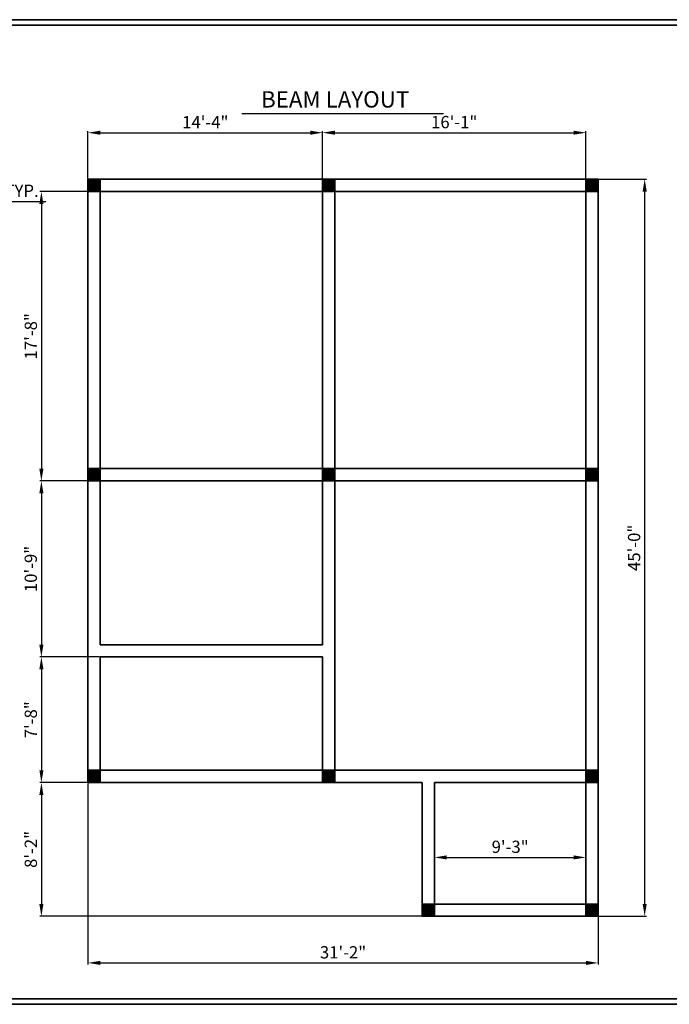
# Model space of a CAD drawing. Units: inches. Extents: x 2396 to 4051, y 1419 to 2191.
# Tile 6 of 7: x 2981 to 3457, y 1470 to 2191. Entities that reach past the tile are written whole.
import ezdxf

# ---------------------------------------------------------------- set-up
doc = ezdxf.new("R2010")
doc.units = ezdxf.units.IN
for name, color, linetype, lineweight in [('A-ANNO-TITL', 7, 'Continuous', 25), ('A-ANNO-TTLB', 7, 'Continuous', 35), ('S-ANNO-DIMS', 2, 'Continuous', 18), ('S-BEAM', 7, 'Continuous', 35)]:
    doc.layers.add(name, color=color, linetype=linetype, lineweight=lineweight)
doc.layers.add('S-COLS', color=242, linetype='Continuous', lineweight=35, true_color=0xcd2027)
doc.styles.get("Standard").update_dxf_attribs({"font": 'arial.ttf'})
doc.dimstyles.new('ISO-25', dxfattribs={"dimtxt": 9, "dimasz": 9, "dimexe": 1.25, "dimexo": 0.625, "dimgap": 2, "dimtad": 1, "dimdec": 1, "dimlunit": 4, "dimtxsty": 'Standard', "dimcen": 2.5, "dimadec": 0, "dimazin": 0, "dimtfac": 1, "dimtdec": 1, "dimtmove": 0, "dimatfit": 3, "dimfxl": 1, "dimarcsym": 0})

# ---------------------------------------------------------------- blocks, each defined once
blk = doc.blocks.new('COL-9X9')
h = blk.add_hatch(color=256)
h.dxf.hatch_style = 1
h.paths.add_polyline_path([(9, 9), (0, 9), (0, 0), (9, 0)])
blk.add_lwpolyline([(0, 9), (9, 9), (9, 0), (0, 0)], close=True)
blk = doc.blocks.new('*D42')
at = {"layer": 'Defpoints', "color": 0, "transparency": 16777216}
for p in [(2809.48, 2065.3), (2857.48, 2065.3), (2857.48, 2058.1)]:
    blk.add_point(p, dxfattribs=at)
at = {"layer": 'S-ANNO-DIMS', "color": 0, "lineweight": -2, "transparency": 16777216}
for p, q in [((2809.48, 2064.68), (2809.48, 2056.85)), ((2857.48, 2064.68), (2857.48, 2056.85)), ((2818.48, 2058.1), (2848.48, 2058.1)), ((2857.48, 2058.1), (2999.73, 2058.1))]:
    blk.add_line(p, q, dxfattribs=at)
at = {"layer": 'S-ANNO-DIMS', "color": 0, "transparency": 16777216}
for points in [[(2818.48, 2059.6), (2818.48, 2056.6), (2809.48, 2058.1)], [(2848.48, 2059.6), (2848.48, 2056.6), (2857.48, 2058.1)]]:
    blk.add_solid(points, dxfattribs=at)
at = {"layer": 'S-ANNO-DIMS', "color": 0, "transparency": 16777216, "insert": (2933.11, 2064.76), "char_height": 9, "attachment_point": 5}
blk.add_mtext('WINDOW W 4\'-0" TYP.', dxfattribs=at)
blk = doc.blocks.new('*D100')
at = {"layer": 'Defpoints', "color": 0, "transparency": 16777216}
for p in [(3030.66, 1632.3), (3404.66, 1534.3), (3404.66, 1500.15)]:
    blk.add_point(p, dxfattribs=at)
at = {"layer": 'S-ANNO-DIMS', "color": 0, "lineweight": -2, "transparency": 16777216}
for p, q in [((3030.66, 1631.68), (3030.66, 1498.9)), ((3404.66, 1533.68), (3404.66, 1498.9)), ((3039.66, 1500.15), (3395.66, 1500.15))]:
    blk.add_line(p, q, dxfattribs=at)
at = {"layer": 'S-ANNO-DIMS', "color": 0, "transparency": 16777216}
for points in [[(3039.66, 1501.65), (3039.66, 1498.65), (3030.66, 1500.15)], [(3395.66, 1501.65), (3395.66, 1498.65), (3404.66, 1500.15)]]:
    blk.add_solid(points, dxfattribs=at)
at = {"layer": 'S-ANNO-DIMS', "color": 0, "transparency": 16777216, "insert": (3217.66, 1506.75), "char_height": 9, "attachment_point": 5}
blk.add_mtext('31\'-2"', dxfattribs=at)
blk = doc.blocks.new('*D101')
at = {"layer": 'Defpoints', "color": 0, "transparency": 16777216}
for p in [(3404.66, 2074.3), (3438.81, 2074.3), (3404.66, 1534.3)]:
    blk.add_point(p, dxfattribs=at)
at = {"layer": 'S-ANNO-DIMS', "color": 0, "lineweight": -2, "transparency": 16777216}
for p, q in [((3405.28, 2074.3), (3440.06, 2074.3)), ((3438.81, 1543.3), (3438.81, 2065.3)), ((3405.28, 1534.3), (3440.06, 1534.3))]:
    blk.add_line(p, q, dxfattribs=at)
at = {"layer": 'S-ANNO-DIMS', "color": 0, "transparency": 16777216}
for points in [[(3437.31, 2065.3), (3440.31, 2065.3), (3438.81, 2074.3)], [(3437.31, 1543.3), (3440.31, 1543.3), (3438.81, 1534.3)]]:
    blk.add_solid(points, dxfattribs=at)
at = {"layer": 'S-ANNO-DIMS', "color": 0, "transparency": 16777216, "insert": (3432.21, 1804.3), "char_height": 9, "attachment_point": 5, "rotation": 90}
blk.add_mtext('45\'-0"', dxfattribs=at)
blk = doc.blocks.new('*D102')
at = {"layer": 'Defpoints', "color": 0, "transparency": 16777216}
for p in [(3202.66, 2108.45), (3030.66, 2074.3), (3202.66, 2074.3)]:
    blk.add_point(p, dxfattribs=at)
at = {"layer": 'S-ANNO-DIMS', "color": 0, "lineweight": -2, "transparency": 16777216}
for p, q in [((3030.66, 2074.93), (3030.66, 2109.7)), ((3039.66, 2108.45), (3193.66, 2108.45)), ((3202.66, 2074.93), (3202.66, 2109.7))]:
    blk.add_line(p, q, dxfattribs=at)
at = {"layer": 'S-ANNO-DIMS', "color": 0, "transparency": 16777216}
for points in [[(3039.66, 2109.95), (3039.66, 2106.95), (3030.66, 2108.45)], [(3193.66, 2109.95), (3193.66, 2106.95), (3202.66, 2108.45)]]:
    blk.add_solid(points, dxfattribs=at)
at = {"layer": 'S-ANNO-DIMS', "color": 0, "transparency": 16777216, "insert": (3116.66, 2114.97), "char_height": 9, "attachment_point": 5}
blk.add_mtext('14\'-4"', dxfattribs=at)
blk = doc.blocks.new('*D103')
at = {"layer": 'Defpoints', "color": 0, "transparency": 16777216}
for p in [(3395.66, 2108.45), (3202.66, 2074.3), (3395.66, 2074.3)]:
    blk.add_point(p, dxfattribs=at)
at = {"layer": 'S-ANNO-DIMS', "color": 0, "lineweight": -2, "transparency": 16777216}
for p, q in [((3202.66, 2074.93), (3202.66, 2109.7)), ((3211.66, 2108.45), (3386.66, 2108.45)), ((3395.66, 2074.93), (3395.66, 2109.7))]:
    blk.add_line(p, q, dxfattribs=at)
at = {"layer": 'S-ANNO-DIMS', "color": 0, "transparency": 16777216}
for points in [[(3211.66, 2109.95), (3211.66, 2106.95), (3202.66, 2108.45)], [(3386.66, 2109.95), (3386.66, 2106.95), (3395.66, 2108.45)]]:
    blk.add_solid(points, dxfattribs=at)
at = {"layer": 'S-ANNO-DIMS', "color": 0, "transparency": 16777216, "insert": (3299.16, 2115.05), "char_height": 9, "attachment_point": 5}
blk.add_mtext('16\'-1"', dxfattribs=at)
blk = doc.blocks.new('*D104')
at = {"layer": 'Defpoints', "color": 0, "transparency": 16777216}
for p in [(3030.66, 2065.3), (2996.51, 1853.3), (3030.66, 1853.3)]:
    blk.add_point(p, dxfattribs=at)
at = {"layer": 'S-ANNO-DIMS', "color": 0, "lineweight": -2, "transparency": 16777216}
for p, q in [((3030.03, 2065.3), (2995.26, 2065.3)), ((2996.51, 2056.3), (2996.51, 1862.3)), ((3030.03, 1853.3), (2995.26, 1853.3))]:
    blk.add_line(p, q, dxfattribs=at)
at = {"layer": 'S-ANNO-DIMS', "color": 0, "transparency": 16777216}
for points in [[(2995.01, 2056.3), (2998.01, 2056.3), (2996.51, 2065.3)], [(2995.01, 1862.3), (2998.01, 1862.3), (2996.51, 1853.3)]]:
    blk.add_solid(points, dxfattribs=at)
at = {"layer": 'S-ANNO-DIMS', "color": 0, "transparency": 16777216, "insert": (2989.91, 1959.3), "char_height": 9, "attachment_point": 5, "rotation": 90}
blk.add_mtext('17\'-8"', dxfattribs=at)
blk = doc.blocks.new('*D105')
at = {"layer": 'Defpoints', "color": 0, "transparency": 16777216}
for p in [(3030.66, 1853.3), (2996.51, 1724.3), (3039.66, 1724.3)]:
    blk.add_point(p, dxfattribs=at)
at = {"layer": 'S-ANNO-DIMS', "color": 0, "lineweight": -2, "transparency": 16777216}
for p, q in [((3030.03, 1853.3), (2995.26, 1853.3)), ((2996.51, 1844.3), (2996.51, 1733.3)), ((3039.03, 1724.3), (2995.26, 1724.3))]:
    blk.add_line(p, q, dxfattribs=at)
at = {"layer": 'S-ANNO-DIMS', "color": 0, "transparency": 16777216}
for points in [[(2995.01, 1844.3), (2998.01, 1844.3), (2996.51, 1853.3)], [(2995.01, 1733.3), (2998.01, 1733.3), (2996.51, 1724.3)]]:
    blk.add_solid(points, dxfattribs=at)
at = {"layer": 'S-ANNO-DIMS', "color": 0, "transparency": 16777216, "insert": (2989.91, 1788.8), "char_height": 9, "attachment_point": 5, "rotation": 90}
blk.add_mtext('10\'-9"', dxfattribs=at)
blk = doc.blocks.new('*D106')
at = {"layer": 'Defpoints', "color": 0, "transparency": 16777216}
for p in [(3039.66, 1724.3), (2996.51, 1632.3), (3030.66, 1632.3)]:
    blk.add_point(p, dxfattribs=at)
at = {"layer": 'S-ANNO-DIMS', "color": 0, "lineweight": -2, "transparency": 16777216}
for p, q in [((3039.03, 1724.3), (2995.26, 1724.3)), ((2996.51, 1715.3), (2996.51, 1641.3)), ((3030.03, 1632.3), (2995.26, 1632.3))]:
    blk.add_line(p, q, dxfattribs=at)
at = {"layer": 'S-ANNO-DIMS', "color": 0, "transparency": 16777216}
for points in [[(2995.01, 1715.3), (2998.01, 1715.3), (2996.51, 1724.3)], [(2995.01, 1641.3), (2998.01, 1641.3), (2996.51, 1632.3)]]:
    blk.add_solid(points, dxfattribs=at)
at = {"layer": 'S-ANNO-DIMS', "color": 0, "transparency": 16777216, "insert": (2989.91, 1678.3), "char_height": 9, "attachment_point": 5, "rotation": 90}
blk.add_mtext('7\'-8"', dxfattribs=at)
blk = doc.blocks.new('*D107')
at = {"layer": 'Defpoints', "color": 0, "transparency": 16777216}
for p in [(3030.66, 1632.3), (2996.51, 1534.3), (3275.66, 1534.3)]:
    blk.add_point(p, dxfattribs=at)
at = {"layer": 'S-ANNO-DIMS', "color": 0, "lineweight": -2, "transparency": 16777216}
for p, q in [((3030.03, 1632.3), (2995.26, 1632.3)), ((2996.51, 1623.3), (2996.51, 1543.3)), ((3275.03, 1534.3), (2995.26, 1534.3))]:
    blk.add_line(p, q, dxfattribs=at)
at = {"layer": 'S-ANNO-DIMS', "color": 0, "transparency": 16777216}
for points in [[(2995.01, 1623.3), (2998.01, 1623.3), (2996.51, 1632.3)], [(2995.01, 1543.3), (2998.01, 1543.3), (2996.51, 1534.3)]]:
    blk.add_solid(points, dxfattribs=at)
at = {"layer": 'S-ANNO-DIMS', "color": 0, "transparency": 16777216, "insert": (2989.91, 1583.3), "char_height": 9, "attachment_point": 5, "rotation": 90}
blk.add_mtext('8\'-2"', dxfattribs=at)
blk = doc.blocks.new('*D108')
at = {"layer": 'Defpoints', "color": 0, "transparency": 16777216}
for p in [(3395.66, 1577.45), (3284.66, 1543.3), (3395.66, 1543.3)]:
    blk.add_point(p, dxfattribs=at)
at = {"layer": 'S-ANNO-DIMS', "color": 0, "lineweight": -2, "transparency": 16777216}
for p, q in [((3284.66, 1543.93), (3284.66, 1578.7)), ((3293.66, 1577.45), (3386.66, 1577.45)), ((3395.66, 1543.93), (3395.66, 1578.7))]:
    blk.add_line(p, q, dxfattribs=at)
at = {"layer": 'S-ANNO-DIMS', "color": 0, "transparency": 16777216}
for points in [[(3293.66, 1578.95), (3293.66, 1575.95), (3284.66, 1577.45)], [(3386.66, 1578.95), (3386.66, 1575.95), (3395.66, 1577.45)]]:
    blk.add_solid(points, dxfattribs=at)
at = {"layer": 'S-ANNO-DIMS', "color": 0, "transparency": 16777216, "insert": (3340.16, 1584.05), "char_height": 9, "attachment_point": 5}
blk.add_mtext('9\'-3"', dxfattribs=at)

msp = doc.modelspace()

# ---------------------------------------------------------------- linework, layer by layer
at = {"layer": 'A-ANNO-TITL'}
msp.add_line((3143.34, 2122.61), (3291.34, 2122.61), dxfattribs=at)
at = {"layer": 'A-ANNO-TTLB'}
for points in [[(2460.66, 2191.26), (4051.21, 2191.26), (4051.21, 1469.82), (2460.66, 1469.82)], [(2464.66, 2187.26), (4047.21, 2187.26), (4047.21, 1473.82), (2464.66, 1473.82)]]:
    msp.add_lwpolyline(points, close=True, dxfattribs=at)
at = {"layer": 'S-BEAM'}
for p, q in [((3030.66, 2074.3), (3404.66, 2074.3)), ((3030.66, 1632.3), (3030.66, 2074.3)), ((3404.66, 2074.3), (3404.66, 1534.3)), ((3039.66, 2065.3), (3202.66, 2065.3)), ((3039.66, 2065.3), (3202.66, 2065.3)), ((3039.66, 1733.3), (3039.66, 2065.3)), ((3039.66, 1921.3), (3039.66, 2065.3)), ((3202.66, 2065.3), (3202.66, 1733.3)), ((3207.66, 2065.3), (3216.66, 2065.3)), ((3207.66, 2065.3), (3395.66, 2065.3)), ((3211.66, 2065.3), (3268.66, 2065.3)), ((3211.66, 2065.3), (3211.66, 1641.3)), ((3395.66, 2065.3), (3395.66, 1853.3)), ((3395.66, 1917.3), (3395.66, 1641.3)), ((3039.66, 1862.3), (3202.66, 1862.3)), ((3211.66, 1862.3), (3395.66, 1862.3)), ((3039.66, 1853.3), (3202.66, 1853.3)), ((3211.66, 1853.3), (3395.66, 1853.3)), ((3202.66, 1733.3), (3039.66, 1733.3)), ((3202.66, 1724.3), (3039.66, 1724.3)), ((3039.66, 1641.3), (3039.66, 1724.3)), ((3202.66, 1724.3), (3202.66, 1641.3)), ((3395.66, 1641.3), (3039.66, 1641.3)), ((3202.66, 1641.3), (3200.66, 1641.3)), ((3284.66, 1641.3), (3275.66, 1641.3)), ((3275.66, 1632.3), (3030.66, 1632.3)), ((3211.66, 1632.3), (3200.66, 1632.3)), ((3275.66, 1632.3), (3275.66, 1534.3)), ((3284.66, 1632.3), (3284.66, 1543.3)), ((3395.66, 1632.3), (3284.66, 1632.3)), ((3395.66, 1637.3), (3395.66, 1543.3)), ((3395.66, 1543.3), (3284.66, 1543.3)), ((3404.66, 1534.3), (3275.66, 1534.3))]:
    msp.add_line(p, q, dxfattribs=at)

# ---------------------------------------------------------------- block references
at = {"layer": 'S-COLS'}
for p in [(3030.66, 2065.3), (3202.66, 2065.3), (3395.66, 2065.3), (3030.66, 1853.3), (3202.66, 1853.3), (3395.66, 1853.3), (3030.66, 1632.3), (3202.66, 1632.3), (3395.66, 1632.3), (3275.66, 1534.3), (3395.66, 1534.3)]:
    msp.add_blockref('COL-9X9', p, dxfattribs=at)

# ---------------------------------------------------------------- texts
at = {"layer": 'A-ANNO-TITL', "insert": (3157.56, 2138.87), "char_height": 12, "attachment_point": 1}
msp.add_mtext_dynamic_manual_height_columns('{\\fArial|b1|i0|c0|p34;BEAM LAYOUT }', width=349.2365, gutter_width=12.5, heights=[0], dxfattribs=at)

# ---------------------------------------------------------------- dimensions: what is measured, and where the dimension line sits
at = {"layer": 'S-ANNO-DIMS'}
for base, p1, p2, picture, middle in [((3202.66, 2108.45), (3030.66, 2074.3), (3202.66, 2074.3), '*D102', (3116.66, 2114.97)), ((3395.66, 2108.45), (3202.66, 2074.3), (3395.66, 2074.3), '*D103', (3299.16, 2115.05)), ((3404.66, 1500.15), (3030.66, 1632.3), (3404.66, 1534.3), '*D100', (3217.66, 1506.75)), ((3395.66, 1577.45), (3284.66, 1543.3), (3395.66, 1543.3), '*D108', (3340.16, 1584.05))]:
    dim = msp.add_linear_dim(base=base, p1=p1, p2=p2, dimstyle='ISO-25', override={"dimdec": 1, "dimlfac": 1, "dimrnd": 0, "dimzin": 1, "dimdsep": 46, "dimlunit": 4, "dimfrac": 2}, dxfattribs=at)
    dim.commit()
    dim.dimension.update_dxf_attribs({"geometry": picture, "text_midpoint": middle})
dim = msp.add_linear_dim(base=(2857.48, 2058.1), p1=(2809.48, 2065.3), p2=(2857.48, 2065.3), text='WINDOW W <> TYP.', dimstyle='ISO-25', override={"dimdec": 1, "dimlfac": 1, "dimrnd": 0, "dimzin": 1, "dimdsep": 46, "dimlunit": 4, "dimfrac": 2}, dxfattribs=at)
dim.commit()
dim.dimension.update_dxf_attribs({"geometry": '*D42', "text_midpoint": (2933.11, 2064.76)})
for base, p1, p2, picture, middle in [((3438.81, 2074.3), (3404.66, 1534.3), (3404.66, 2074.3), '*D101', (3432.21, 1804.3)), ((2996.51, 1853.3), (3030.66, 2065.3), (3030.66, 1853.3), '*D104', (2989.91, 1959.3)), ((2996.51, 1724.3), (3030.66, 1853.3), (3039.66, 1724.3), '*D105', (2989.91, 1788.8)), ((2996.51, 1632.3), (3039.66, 1724.3), (3030.66, 1632.3), '*D106', (2989.91, 1678.3)), ((2996.51, 1534.3), (3030.66, 1632.3), (3275.66, 1534.3), '*D107', (2989.91, 1583.3))]:
    dim = msp.add_linear_dim(base=base, p1=p1, p2=p2, angle=90, dimstyle='ISO-25', override={"dimdec": 1, "dimlfac": 1, "dimrnd": 0, "dimzin": 1, "dimdsep": 46, "dimlunit": 4, "dimfrac": 2}, dxfattribs=at)
    dim.commit()
    dim.dimension.update_dxf_attribs({"geometry": picture, "text_midpoint": middle})

doc.saveas('drawing.dxf')
